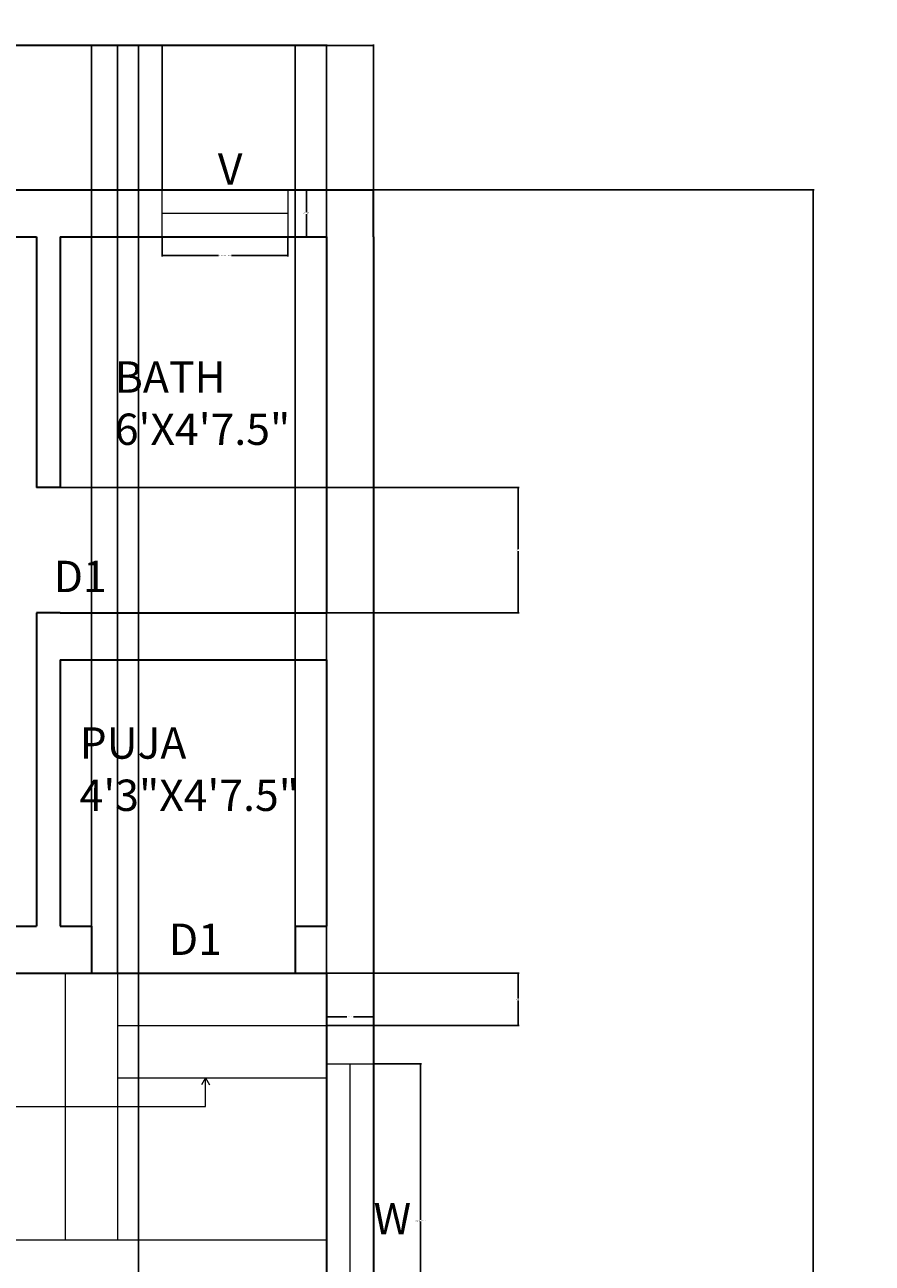
# Model space of a CAD drawing. Units: inches. Extents: x -4347 to -3836, y 955 to 1521.
# Tile 11 of 11: x -3998 to -3836, y 1284 to 1521. Entities that reach past the tile are written whole.
import ezdxf

# ---------------------------------------------------------------- set-up
doc = ezdxf.new("R2010")
doc.units = ezdxf.units.IN
doc.header["$MEASUREMENT"] = 0
for name, color, linetype, lineweight in [('A-ANNO-DIMS', 2, 'Continuous', 18), ('A-ANNO-SYMB', 7, 'Continuous', 18), ('A-ANNO-TEXT', 7, 'Continuous', 18), ('A-AREA-IDEN', 7, 'Continuous', 18), ('A-FLOR-STRS', 7, 'Continuous', 18), ('A-GLAZ', 4, 'Continuous', 18), ('A-WALL', 7, 'Continuous', 35)]:
    doc.layers.add(name, color=color, linetype=linetype, lineweight=lineweight)
doc.styles.get("Standard").update_dxf_attribs({"font": 'arial.ttf'})
doc.dimstyles.get("Standard").update_dxf_attribs({"dimtxt": 0.18, "dimasz": 0.18, "dimexe": 0.18, "dimexo": 0.0625, "dimgap": 0.09, "dimtad": 0, "dimtih": 1, "dimtoh": 1, "dimdec": 0, "dimzin": 0, "dimdsep": 46, "dimlunit": 3, "dimtxsty": 'Standard', "dimcen": 0.09, "dimadec": 0, "dimazin": 0, "dimtfac": 1, "dimtdec": 0, "dimtofl": 0, "dimtmove": 0, "dimatfit": 3, "dimfxl": 1, "dimtolj": 1, "dimtzin": 0, "dimarcsym": 0})

# ---------------------------------------------------------------- blocks, each defined once
blk = doc.blocks.new('*D1')
at = {"layer": 'A-ANNO-DIMS', "color": 0, "lineweight": -2, "transparency": 16777216}
for p, q in [((-4318.58, 1489.85), (-4318.58, 1517.61)), ((-4318.4, 1517.43), (-4135.47, 1517.43)), ((-3931.76, 1517.43), (-4114.69, 1517.43)), ((-3931.58, 1489.85), (-3931.58, 1517.61))]:
    blk.add_line(p, q, dxfattribs=at)
at = {"layer": 'A-ANNO-DIMS', "color": 0, "transparency": 16777216}
for points in [[(-4318.4, 1517.46), (-4318.4, 1517.4), (-4318.58, 1517.43)], [(-3931.76, 1517.46), (-3931.76, 1517.4), (-3931.58, 1517.43)]]:
    blk.add_solid(points, dxfattribs=at)
at = {"layer": 'Defpoints', "color": 0, "transparency": 16777216}
for p in [(-3931.58, 1517.43), (-4318.58, 1489.79), (-3931.58, 1489.79)]:
    blk.add_point(p, dxfattribs=at)
at = {"layer": 'A-ANNO-DIMS', "color": 0, "transparency": 16777216, "insert": (-4125.08, 1517.43), "char_height": 6, "attachment_point": 5}
blk.add_mtext('\\A1;32\'-3"', dxfattribs=at)
blk = doc.blocks.new('*D2')
at = {"layer": 'A-ANNO-DIMS', "color": 0, "lineweight": -2, "transparency": 16777216}
for p, q in [((-3931.52, 1489.79), (-3847.29, 1489.79)), ((-3847.47, 1489.61), (-3847.47, 1245.44)), ((-3847.47, 994.97), (-3847.47, 1239.13)), ((-3931.52, 994.79), (-3847.29, 994.79))]:
    blk.add_line(p, q, dxfattribs=at)
at = {"layer": 'A-ANNO-DIMS', "color": 0, "transparency": 16777216}
for points in [[(-3847.5, 1489.61), (-3847.44, 1489.61), (-3847.47, 1489.79)], [(-3847.5, 994.97), (-3847.44, 994.97), (-3847.47, 994.79)]]:
    blk.add_solid(points, dxfattribs=at)
at = {"layer": 'Defpoints', "color": 0, "transparency": 16777216}
for p in [(-3931.58, 1489.79), (-3931.58, 994.79), (-3847.47, 994.79)]:
    blk.add_point(p, dxfattribs=at)
at = {"layer": 'A-ANNO-DIMS', "color": 0, "transparency": 16777216, "insert": (-3847.47, 1242.29), "char_height": 6, "attachment_point": 5}
blk.add_mtext('\\A1;41\'-3"', dxfattribs=at)
blk = doc.blocks.new('GLAZ-24IN')
for p, q in [((0, 9), (24, 9)), ((0, 0), (0, 9)), ((24, 9), (24, 0)), ((0, 4.5), (24, 4.5)), ((24, 0), (0, 0))]:
    blk.add_line(p, q)
blk = doc.blocks.new('GLAZ-60IN')
for p, q in [((0, 9), (60, 9)), ((0, 0), (0, 9)), ((60, 9), (60, 0)), ((0, 4.5), (60, 4.5)), ((60, 0), (0, 0))]:
    blk.add_line(p, q)
blk = doc.blocks.new('*D24')
at = {"layer": 'A-ANNO-DIMS', "color": 0, "lineweight": -2, "transparency": 16777216}
for p, q in [((-3972.01, 1480.73), (-3972.01, 1477.01)), ((-3948.01, 1480.73), (-3948.01, 1477.01)), ((-3971.83, 1477.19), (-3961.23, 1477.19)), ((-3948.19, 1477.19), (-3958.78, 1477.19))]:
    blk.add_line(p, q, dxfattribs=at)
at = {"layer": 'A-ANNO-DIMS', "color": 0, "transparency": 16777216}
for points in [[(-3971.83, 1477.22), (-3971.83, 1477.16), (-3972.01, 1477.19)], [(-3948.19, 1477.22), (-3948.19, 1477.16), (-3948.01, 1477.19)]]:
    blk.add_solid(points, dxfattribs=at)
at = {"layer": 'Defpoints', "color": 0, "transparency": 16777216}
for p in [(-3972.01, 1480.79), (-3948.01, 1480.79), (-3948.01, 1477.19)]:
    blk.add_point(p, dxfattribs=at)
at = {"layer": 'A-ANNO-DIMS', "color": 0, "transparency": 16777216, "insert": (-3960.01, 1477.19), "char_height": 0.18, "attachment_point": 5}
blk.add_mtext('\\A1;GLAZING 2\'-0" TYP.', dxfattribs=at)
blk = doc.blocks.new('*D25')
at = {"layer": 'A-ANNO-DIMS', "color": 0, "lineweight": -2, "transparency": 16777216}
for p, q in [((-3947.94, 1489.79), (-3944.23, 1489.79)), ((-3944.41, 1489.61), (-3944.41, 1485.47)), ((-3944.41, 1480.97), (-3944.41, 1485.11)), ((-3947.94, 1480.79), (-3944.23, 1480.79))]:
    blk.add_line(p, q, dxfattribs=at)
at = {"layer": 'A-ANNO-DIMS', "color": 0, "transparency": 16777216}
for points in [[(-3944.44, 1489.61), (-3944.38, 1489.61), (-3944.41, 1489.79)], [(-3944.44, 1480.97), (-3944.38, 1480.97), (-3944.41, 1480.79)]]:
    blk.add_solid(points, dxfattribs=at)
at = {"layer": 'Defpoints', "color": 0, "transparency": 16777216}
for p in [(-3948.01, 1489.79), (-3944.41, 1489.79), (-3948.01, 1480.79)]:
    blk.add_point(p, dxfattribs=at)
at = {"layer": 'A-ANNO-DIMS', "color": 0, "transparency": 16777216, "insert": (-3944.41, 1485.29), "char_height": 0.18, "attachment_point": 5}
blk.add_mtext('\\A1;0\'-9" TYP.', dxfattribs=at)
blk = doc.blocks.new('*D28')
at = {"layer": 'A-ANNO-DIMS', "color": 0, "lineweight": -2, "transparency": 16777216}
for p, q in [((-3931.52, 1322.43), (-3922.4, 1322.43)), ((-3922.58, 1322.25), (-3922.58, 1292.61)), ((-3922.58, 1262.61), (-3922.58, 1292.25)), ((-3931.52, 1262.43), (-3922.4, 1262.43))]:
    blk.add_line(p, q, dxfattribs=at)
at = {"layer": 'A-ANNO-DIMS', "color": 0, "transparency": 16777216}
for points in [[(-3922.61, 1322.25), (-3922.55, 1322.25), (-3922.58, 1322.43)], [(-3922.61, 1262.61), (-3922.55, 1262.61), (-3922.58, 1262.43)]]:
    blk.add_solid(points, dxfattribs=at)
at = {"layer": 'Defpoints', "color": 0, "transparency": 16777216}
for p in [(-3931.58, 1322.43), (-3922.58, 1322.43), (-3931.58, 1262.43)]:
    blk.add_point(p, dxfattribs=at)
at = {"layer": 'A-ANNO-DIMS', "color": 0, "transparency": 16777216, "insert": (-3922.58, 1292.43), "char_height": 0.18, "attachment_point": 5}
blk.add_mtext('\\A1;GLAZING 5\'-0" TYP.', dxfattribs=at)
blk = doc.blocks.new('*D29')
at = {"layer": 'A-ANNO-DIMS', "color": 0, "lineweight": -2, "transparency": 16777216}
for p, q in [((-3940.58, 1322.49), (-3940.58, 1331.61)), ((-3940.4, 1331.43), (-3936.72, 1331.43)), ((-3931.76, 1331.43), (-3935.44, 1331.43)), ((-3931.58, 1322.49), (-3931.58, 1331.61))]:
    blk.add_line(p, q, dxfattribs=at)
at = {"layer": 'A-ANNO-DIMS', "color": 0, "transparency": 16777216}
for points in [[(-3940.4, 1331.46), (-3940.4, 1331.4), (-3940.58, 1331.43)], [(-3931.76, 1331.46), (-3931.76, 1331.4), (-3931.58, 1331.43)]]:
    blk.add_solid(points, dxfattribs=at)
at = {"layer": 'Defpoints', "color": 0, "transparency": 16777216}
for p in [(-3940.58, 1331.43), (-3940.58, 1322.43), (-3931.58, 1322.43)]:
    blk.add_point(p, dxfattribs=at)
at = {"layer": 'A-ANNO-DIMS', "color": 0, "transparency": 16777216, "insert": (-3936.08, 1331.43), "char_height": 0.18, "attachment_point": 5}
blk.add_mtext('\\A1;0\'-9" TYP.', dxfattribs=at)
blk = doc.blocks.new('*D38')
at = {"layer": 'A-ANNO-DIMS', "color": 0, "lineweight": -2, "transparency": 16777216}
for p, q in [((-4057.8, 1489.85), (-4057.8, 1517.62)), ((-4057.62, 1517.44), (-4015.23, 1517.44)), ((-3972.19, 1517.44), (-4014.57, 1517.44)), ((-3972.01, 1489.85), (-3972.01, 1517.62))]:
    blk.add_line(p, q, dxfattribs=at)
at = {"layer": 'A-ANNO-DIMS', "color": 0, "transparency": 16777216}
for points in [[(-4057.62, 1517.47), (-4057.62, 1517.41), (-4057.8, 1517.44)], [(-3972.19, 1517.47), (-3972.19, 1517.41), (-3972.01, 1517.44)]]:
    blk.add_solid(points, dxfattribs=at)
at = {"layer": 'Defpoints', "color": 0, "transparency": 16777216}
for p in [(-3972.01, 1517.44), (-4057.8, 1489.79), (-3972.01, 1489.79)]:
    blk.add_point(p, dxfattribs=at)
at = {"layer": 'A-ANNO-DIMS', "color": 0, "transparency": 16777216, "insert": (-4014.9, 1517.44), "char_height": 0.18, "attachment_point": 5}
blk.add_mtext('\\A1;7\'-2"', dxfattribs=at)
blk = doc.blocks.new('*D47')
at = {"layer": 'A-ANNO-DIMS', "color": 0, "lineweight": -2, "transparency": 16777216}
for p, q in [((-4120.58, 1288.73), (-4120.58, 966.96)), ((-3940.58, 1288.73), (-3940.58, 966.96)), ((-4120.4, 967.14), (-4030.97, 967.14)), ((-3940.76, 967.14), (-4030.19, 967.14))]:
    blk.add_line(p, q, dxfattribs=at)
at = {"layer": 'A-ANNO-DIMS', "color": 0, "transparency": 16777216}
for points in [[(-4120.4, 967.17), (-4120.4, 967.11), (-4120.58, 967.14)], [(-3940.76, 967.17), (-3940.76, 967.11), (-3940.58, 967.14)]]:
    blk.add_solid(points, dxfattribs=at)
at = {"layer": 'Defpoints', "color": 0, "transparency": 16777216}
for p in [(-4120.58, 1288.79), (-3940.58, 1288.79), (-3940.58, 967.14)]:
    blk.add_point(p, dxfattribs=at)
at = {"layer": 'A-ANNO-DIMS', "color": 0, "transparency": 16777216, "insert": (-4030.58, 967.14), "char_height": 0.18, "attachment_point": 5}
blk.add_mtext('\\A1;15\'-0"', dxfattribs=at)
blk = doc.blocks.new('*D50')
at = {"layer": 'A-ANNO-DIMS', "color": 0, "lineweight": -2, "transparency": 16777216}
for p, q in [((-3980.58, 1339.85), (-3980.58, 1517.62)), ((-3980.4, 1517.44), (-3960.91, 1517.44)), ((-3940.76, 1517.44), (-3960.25, 1517.44)), ((-3940.58, 1339.85), (-3940.58, 1517.62))]:
    blk.add_line(p, q, dxfattribs=at)
at = {"layer": 'A-ANNO-DIMS', "color": 0, "transparency": 16777216}
for points in [[(-3980.4, 1517.47), (-3980.4, 1517.41), (-3980.58, 1517.44)], [(-3940.76, 1517.47), (-3940.76, 1517.41), (-3940.58, 1517.44)]]:
    blk.add_solid(points, dxfattribs=at)
at = {"layer": 'Defpoints', "color": 0, "transparency": 16777216}
for p in [(-3940.58, 1517.44), (-3980.58, 1339.79), (-3940.58, 1339.79)]:
    blk.add_point(p, dxfattribs=at)
at = {"layer": 'A-ANNO-DIMS', "color": 0, "transparency": 16777216, "insert": (-3960.58, 1517.44), "char_height": 0.18, "attachment_point": 5}
blk.add_mtext('\\A1;3\'-4"', dxfattribs=at)
blk = doc.blocks.new('*D51')
at = {"layer": 'A-ANNO-DIMS', "color": 0, "lineweight": -2, "transparency": 16777216}
for p, q in [((-3940.52, 1339.79), (-3903.75, 1339.79)), ((-3903.93, 1339.61), (-3903.93, 1334.97)), ((-3903.93, 1329.97), (-3903.93, 1334.61)), ((-3940.52, 1329.79), (-3903.75, 1329.79))]:
    blk.add_line(p, q, dxfattribs=at)
at = {"layer": 'A-ANNO-DIMS', "color": 0, "transparency": 16777216}
for points in [[(-3903.96, 1339.61), (-3903.9, 1339.61), (-3903.93, 1339.79)], [(-3903.96, 1329.97), (-3903.9, 1329.97), (-3903.93, 1329.79)]]:
    blk.add_solid(points, dxfattribs=at)
at = {"layer": 'Defpoints', "color": 0, "transparency": 16777216}
for p in [(-3940.58, 1339.79), (-3940.58, 1329.79), (-3903.93, 1329.79)]:
    blk.add_point(p, dxfattribs=at)
at = {"layer": 'A-ANNO-DIMS', "color": 0, "transparency": 16777216, "insert": (-3903.93, 1334.79), "char_height": 0.18, "attachment_point": 5}
blk.add_mtext('\\A1;0\'-10"', dxfattribs=at)
blk = doc.blocks.new('*D53')
at = {"layer": 'A-ANNO-DIMS', "color": 0, "lineweight": -2, "transparency": 16777216}
for p, q in [((-3976.58, 1135.85), (-3976.58, 1517.62)), ((-3976.4, 1517.44), (-3958.91, 1517.44)), ((-3940.76, 1517.44), (-3958.25, 1517.44)), ((-3940.58, 1135.85), (-3940.58, 1517.62))]:
    blk.add_line(p, q, dxfattribs=at)
at = {"layer": 'A-ANNO-DIMS', "color": 0, "transparency": 16777216}
for points in [[(-3976.4, 1517.47), (-3976.4, 1517.41), (-3976.58, 1517.44)], [(-3940.76, 1517.47), (-3940.76, 1517.41), (-3940.58, 1517.44)]]:
    blk.add_solid(points, dxfattribs=at)
at = {"layer": 'Defpoints', "color": 0, "transparency": 16777216}
for p in [(-3940.58, 1517.44), (-3976.58, 1135.79), (-3940.58, 1135.79)]:
    blk.add_point(p, dxfattribs=at)
at = {"layer": 'A-ANNO-DIMS', "color": 0, "transparency": 16777216, "insert": (-3958.58, 1517.44), "char_height": 0.18, "attachment_point": 5}
blk.add_mtext('\\A1;3\'-0"', dxfattribs=at)
blk = doc.blocks.new('*D57')
at = {"layer": 'A-ANNO-DIMS', "color": 0, "lineweight": -2, "transparency": 16777216}
for p, q in [((-3985.58, 1348.85), (-3985.58, 1517.62)), ((-3985.4, 1517.44), (-3966.41, 1517.44)), ((-3946.76, 1517.44), (-3965.75, 1517.44)), ((-3946.58, 1348.85), (-3946.58, 1517.62))]:
    blk.add_line(p, q, dxfattribs=at)
at = {"layer": 'A-ANNO-DIMS', "color": 0, "transparency": 16777216}
for points in [[(-3985.4, 1517.47), (-3985.4, 1517.41), (-3985.58, 1517.44)], [(-3946.76, 1517.47), (-3946.76, 1517.41), (-3946.58, 1517.44)]]:
    blk.add_solid(points, dxfattribs=at)
at = {"layer": 'Defpoints', "color": 0, "transparency": 16777216}
for p in [(-3946.58, 1517.44), (-3985.58, 1348.79), (-3946.58, 1348.79)]:
    blk.add_point(p, dxfattribs=at)
at = {"layer": 'A-ANNO-DIMS', "color": 0, "transparency": 16777216, "insert": (-3966.08, 1517.44), "char_height": 0.18, "attachment_point": 5}
blk.add_mtext('\\A1;3\'-3"', dxfattribs=at)
blk = doc.blocks.new('*D59')
at = {"layer": 'A-ANNO-DIMS', "color": 0, "lineweight": -2, "transparency": 16777216}
for p, q in [((-3991.52, 1432.79), (-3903.75, 1432.79)), ((-3903.93, 1432.61), (-3903.93, 1420.97)), ((-3903.93, 1408.97), (-3903.93, 1420.61)), ((-3991.52, 1408.79), (-3903.75, 1408.79))]:
    blk.add_line(p, q, dxfattribs=at)
at = {"layer": 'A-ANNO-DIMS', "color": 0, "transparency": 16777216}
for points in [[(-3903.96, 1432.61), (-3903.9, 1432.61), (-3903.93, 1432.79)], [(-3903.96, 1408.97), (-3903.9, 1408.97), (-3903.93, 1408.79)]]:
    blk.add_solid(points, dxfattribs=at)
at = {"layer": 'Defpoints', "color": 0, "transparency": 16777216}
for p in [(-3991.58, 1432.79), (-3903.93, 1432.79), (-3991.58, 1408.79)]:
    blk.add_point(p, dxfattribs=at)
at = {"layer": 'A-ANNO-DIMS', "color": 0, "transparency": 16777216, "insert": (-3903.93, 1420.79), "char_height": 0.18, "attachment_point": 5}
blk.add_mtext('\\A1;2\'-0"', dxfattribs=at)

msp = doc.modelspace()

# ---------------------------------------------------------------- linework, layer by layer
at = {"layer": 'A-ANNO-SYMB'}
for p, q in [((-3963.77, 1319.79), (-3964.52, 1318.45)), ((-3963.77, 1314.29), (-3963.77, 1319.79)), ((-3963.77, 1319.79), (-3963.01, 1318.45)), ((-4120.58, 1314.29), (-3963.77, 1314.29))]:
    msp.add_line(p, q, dxfattribs=at)
at = {"layer": 'A-FLOR-STRS'}
for p, q in [((-3990.58, 1339.79), (-3990.58, 1288.79)), ((-3980.58, 1339.79), (-3980.58, 1288.79)), ((-3980.58, 1329.79), (-3980.58, 1319.79)), ((-3980.58, 1329.79), (-3940.58, 1329.79)), ((-3980.58, 1319.79), (-3940.58, 1319.79)), ((-4120.58, 1288.79), (-3940.58, 1288.79))]:
    msp.add_line(p, q, dxfattribs=at)
at = {"layer": 'A-WALL'}
for p, q in [((-4318.58, 1489.79), (-3931.58, 1489.79)), ((-3931.58, 1480.79), (-3931.58, 1489.79)), ((-4108.58, 1480.79), (-3996.08, 1480.79)), ((-3996.08, 1480.79), (-3996.08, 1432.79)), ((-3991.58, 1480.79), (-3991.58, 1432.79)), ((-3991.58, 1480.79), (-3940.58, 1480.79)), ((-3940.58, 1480.79), (-3940.58, 1408.79)), ((-3931.58, 1480.79), (-3931.58, 994.79)), ((-3991.58, 1432.79), (-3996.08, 1432.79)), ((-3991.58, 1408.79), (-3996.08, 1408.79)), ((-3996.08, 1408.79), (-3996.08, 1348.79)), ((-3991.58, 1408.79), (-3940.58, 1408.79)), ((-3991.58, 1399.79), (-3940.58, 1399.79)), ((-3991.58, 1399.79), (-3991.58, 1348.79)), ((-3940.58, 1399.79), (-3940.58, 1348.79)), ((-4120.58, 1348.79), (-3996.08, 1348.79)), ((-3991.58, 1348.79), (-3985.58, 1348.79)), ((-3985.58, 1348.79), (-3985.58, 1339.79)), ((-3946.58, 1348.79), (-3946.58, 1339.79)), ((-3946.58, 1348.79), (-3940.58, 1348.79)), ((-4120.58, 1339.79), (-3940.58, 1339.79)), ((-3940.58, 1339.79), (-3940.58, 1135.79))]:
    msp.add_line(p, q, dxfattribs=at)

# ---------------------------------------------------------------- block references
at = {"layer": 'A-GLAZ'}
msp.add_blockref('GLAZ-24IN', (-3972.01, 1480.79), dxfattribs=at)
at = {"layer": 'A-GLAZ', "rotation": 90.00000000000007}
msp.add_blockref('GLAZ-60IN', (-3931.58, 1262.43), dxfattribs=at)

# ---------------------------------------------------------------- texts
at = {"layer": 'A-ANNO-TEXT', "char_height": 6, "attachment_point": 1}
for s, insert in [('V', (-3961.38, 1496.74)), ('D1', (-3992.81, 1418.76)), ('W', (-3931.58, 1295.82))]:
    msp.add_mtext(s, dxfattribs=dict(at, insert=insert))
at = {"layer": 'A-ANNO-TEXT', "insert": (-3970.78, 1349.3), "char_height": 6, "attachment_point": 1}
msp.add_mtext_dynamic_manual_height_columns('D1', width=0.1927, gutter_width=1, heights=[0], dxfattribs=at)
at = {"layer": 'A-AREA-IDEN', "char_height": 6, "attachment_point": 1}
for s, insert in [('BATH\\P6\'X4\'7.5"', (-3981.1, 1456.94)), ('PUJA\\P4\'3"X4\'7.5"', (-3987.84, 1386.87))]:
    msp.add_mtext(s, dxfattribs=dict(at, insert=insert))

# ---------------------------------------------------------------- dimensions: what is measured, and where the dimension line sits
at = {"layer": 'A-ANNO-DIMS'}
for base, p1, p2, override, picture, middle in [((-3931.58, 1517.43), (-4318.58, 1489.79), (-3931.58, 1489.79), {"dimtxt": 6, "dimclrd": 0, "dimclre": 0, "dimclrt": 0}, '*D1', (-4125.08, 1517.43)), ((-3972.01, 1517.44), (-4057.8, 1489.79), (-3972.01, 1489.79), {"dimdec": 1, "dimlfac": 1, "dimrnd": 0, "dimzin": 1, "dimdsep": 46, "dimlunit": 4, "dimfrac": 2}, '*D38', (-4014.9, 1517.44)), ((-3946.58, 1517.44), (-3985.58, 1348.79), (-3946.58, 1348.79), {"dimdec": 1, "dimlfac": 1, "dimrnd": 0, "dimzin": 1, "dimdsep": 46, "dimlunit": 4, "dimfrac": 2}, '*D57', (-3966.08, 1517.44)), ((-3940.58, 1517.44), (-3980.58, 1339.79), (-3940.58, 1339.79), {"dimdec": 1, "dimlfac": 1, "dimrnd": 0, "dimzin": 1, "dimdsep": 46, "dimlunit": 4, "dimfrac": 2}, '*D50', (-3960.58, 1517.44)), ((-3940.58, 1517.44), (-3976.58, 1135.79), (-3940.58, 1135.79), {"dimdec": 1, "dimlfac": 1, "dimrnd": 0, "dimzin": 1, "dimdsep": 46, "dimlunit": 4, "dimfrac": 2}, '*D53', (-3958.58, 1517.44)), ((-3940.58, 967.14), (-4120.58, 1288.79), (-3940.58, 1288.79), {"dimdec": 1, "dimlfac": 1, "dimrnd": 0, "dimzin": 1, "dimdsep": 46, "dimlunit": 4, "dimfrac": 2}, '*D47', (-4030.58, 967.14))]:
    dim = msp.add_linear_dim(base=base, p1=p1, p2=p2, dimstyle='Standard', override=override, dxfattribs=at)
    dim.commit()
    dim.dimension.update_dxf_attribs({"geometry": picture, "text_midpoint": middle})
for base, p1, p2, angle, text, picture, middle in [((-3944.41, 1489.79), (-3948.01, 1480.79), (-3948.01, 1489.79), 90, '<> TYP.', '*D25', (-3944.41, 1485.29)), ((-3940.58, 1331.43), (-3931.58, 1322.43), (-3940.58, 1322.43), 180, '<> TYP.', '*D29', (-3936.08, 1331.43)), ((-3922.58, 1322.43), (-3931.58, 1262.43), (-3931.58, 1322.43), 90, 'GLAZING <> TYP.', '*D28', (-3922.58, 1292.43))]:
    dim = msp.add_linear_dim(base=base, p1=p1, p2=p2, angle=angle, text=text, dimstyle='Standard', override={"dimdec": 1, "dimlfac": 1, "dimrnd": 0, "dimzin": 1, "dimdsep": 46, "dimlunit": 4, "dimfrac": 2}, dxfattribs=at)
    dim.commit()
    dim.dimension.update_dxf_attribs({"geometry": picture, "text_midpoint": middle})
for base, p1, p2, override, picture, middle in [((-3847.47, 994.79), (-3931.58, 1489.79), (-3931.58, 994.79), {"dimtxt": 6, "dimclrd": 0, "dimclre": 0, "dimclrt": 0}, '*D2', (-3847.47, 1242.29)), ((-3903.93, 1432.79), (-3991.58, 1408.79), (-3991.58, 1432.79), {"dimdec": 1, "dimlfac": 1, "dimrnd": 0, "dimzin": 1, "dimdsep": 46, "dimlunit": 4, "dimfrac": 2}, '*D59', (-3903.93, 1420.79)), ((-3903.93, 1329.79), (-3940.58, 1339.79), (-3940.58, 1329.79), {"dimdec": 1, "dimlfac": 1, "dimrnd": 0, "dimzin": 1, "dimdsep": 46, "dimlunit": 4, "dimfrac": 2}, '*D51', (-3903.93, 1334.79))]:
    dim = msp.add_linear_dim(base=base, p1=p1, p2=p2, angle=90, dimstyle='Standard', override=override, dxfattribs=at)
    dim.commit()
    dim.dimension.update_dxf_attribs({"geometry": picture, "text_midpoint": middle})
dim = msp.add_linear_dim(base=(-3948.01, 1477.19), p1=(-3972.01, 1480.79), p2=(-3948.01, 1480.79), text='GLAZING <> TYP.', dimstyle='Standard', override={"dimdec": 1, "dimlfac": 1, "dimrnd": 0, "dimzin": 1, "dimdsep": 46, "dimlunit": 4, "dimfrac": 2}, dxfattribs=at)
dim.commit()
dim.dimension.update_dxf_attribs({"geometry": '*D24', "text_midpoint": (-3960.01, 1477.19)})

doc.saveas('drawing.dxf')
